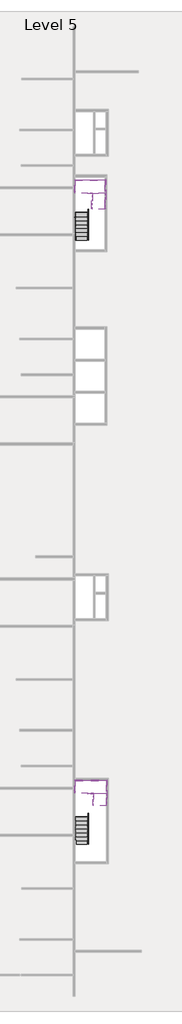
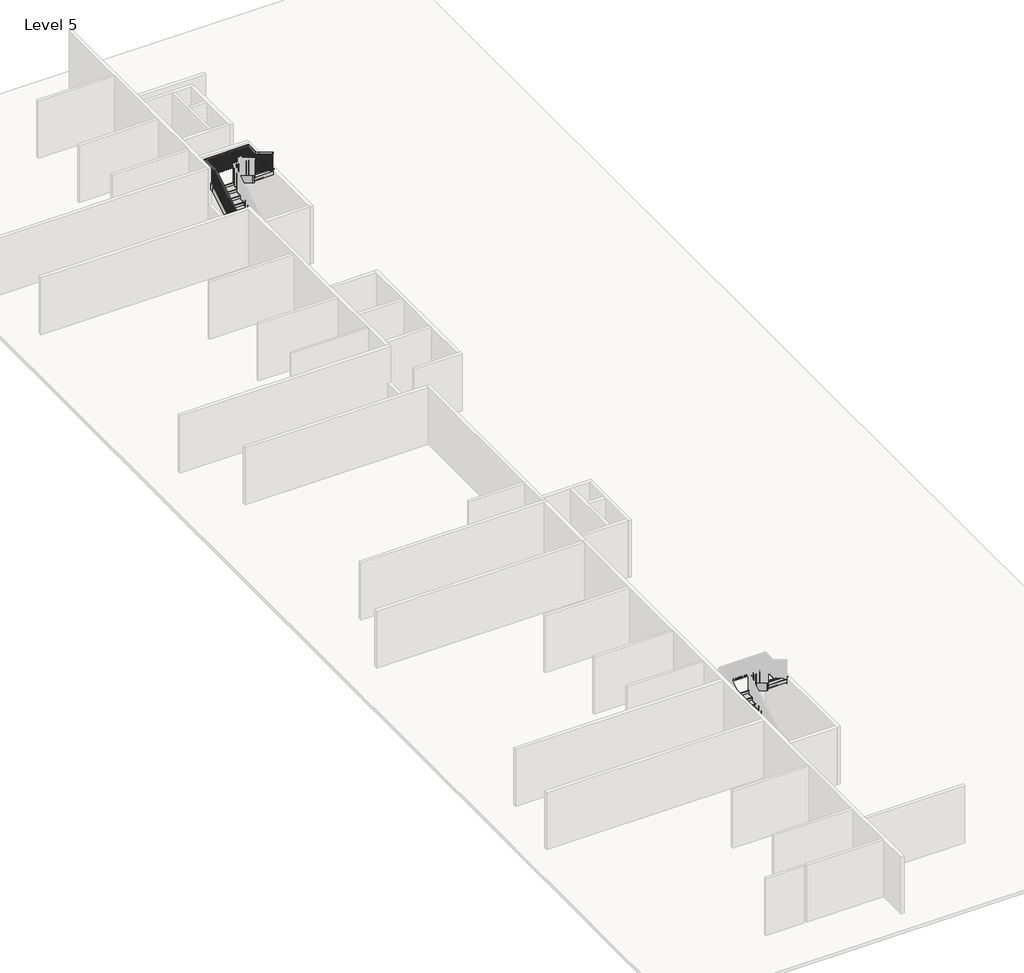
# One storey, part 8 of 8: 16 members, 4 stair flights, 2 slabs, 1 railing.
"""IFC4 building model written with IfcOpenShell, lengths in millimetres."""

from ifc_helpers import new_model, si_unit, frame, origin, place, context, project, spatial, polyline, outline, extrude, faceted_brep, transform, mapped, element, save
from components import non_monolithic_landing_1beb21ea, non_monolithic_landing_abd20321, stair_flight_c80e62dd, stair_flight_f3376f64, stair_flight_9c09f5e7, stair_flight_7705a6e8

model = new_model("IFC4")

# Units and contexts
model_context = context("Model", 3, world=origin())
ifc_project = project(units=[si_unit("LENGTHUNIT", "METRE", prefix="MILLI")], contexts=[model_context])

# Site, building, storey
site = spatial("IfcSite", under=ifc_project)
building = spatial("IfcBuilding", under=site)
storey = spatial("IfcBuildingStorey", under=building, Name="Level 5", Elevation=37426.6172466)

# Members
placement = place(None, origin())
element("IfcMember", 1, ObjectType="Stringer - 2\" Width", at=placement, inside=storey, context=model_context, shape_type="SweptSolid", body=[
    extrude(outline(polyline([(-23154.3851539, 37426.6172466), (-23154.3851539, 37638.7317586), (-19467.0440987, 39873.4839133), (-19381.8896422, 39568.6839133), (-22916.2996422, 37426.6172466), (-23154.3851539, 37426.6172466)])), frame((-3668.2415084, 0.0, 0.0), z_axis=(1.0, 0.0, 0.0), x_axis=(0.0, 1.0, 0.0)), (0.0, 0.0, 1.0), 50.8),
])
element("IfcMember", 2, ObjectType="Stringer - 2\" Width", at=placement, inside=storey, context=model_context, shape_type="SweptSolid", body=[
    extrude(outline(polyline([(-23154.3851539, 37426.6172466), (-23154.3851539, 37638.7317586), (-19572.9851539, 39809.2772131), (-19572.9851539, 39452.8684516), (-22916.2996422, 37426.6172466), (-23154.3851539, 37426.6172466)])), frame((-2703.0415084, 0.0, 0.0), z_axis=(1.0, 0.0, 0.0), x_axis=(0.0, 1.0, 0.0)), (0.0, 0.0, 1.0), 50.8),
])
element("IfcMember", 3, ObjectType="Stringer - 2\" Width", at=placement, inside=storey, context=model_context, shape_type="SweptSolid", body=[
    extrude(outline(polyline([(-19297.9262092, 39873.4839133), (-19383.0806657, 39568.6839133), (-20360.3851539, 40160.9896637), (-20360.3851539, 40517.3984252), (-19297.9262092, 39873.4839133)])), frame((-1382.2415084, 0.0, 0.0), z_axis=(1.0, 0.0, 0.0), x_axis=(0.0, 1.0, 0.0)), (0.0, 0.0, 1.0), 50.8),
])
element("IfcMember", 4, ObjectType="Stringer - 2\" Width", at=placement, inside=storey, context=model_context, shape_type="SweptSolid", body=[
    extrude(outline(polyline([(-19522.1851539, 40009.3984252), (-19522.1851539, 39652.9896637), (-20360.3851539, 40160.9896637), (-20360.3851539, 40517.3984252), (-19522.1851539, 40009.3984252)])), frame((-2347.4415084, 0.0, 0.0), z_axis=(1.0, 0.0, 0.0), x_axis=(0.0, 1.0, 0.0)), (0.0, 0.0, 1.0), 50.8),
])
element("IfcMember", 5, ObjectType="Stringer - 2\" Width", at=placement, inside=storey, context=model_context, shape_type="Brep", body=[
    faceted_brep([(-1382.2415084, -19297.9262092, 39873.4839133), (-1331.4415084, -19297.9262092, 39873.4839133), (-1331.4415084, -18556.9851539, 39873.4839133), (-1382.2415084, -18607.7851539, 39873.4839133), (-1382.2415084, -19383.0806657, 39568.6839133), (-1382.2415084, -18607.7851539, 39568.6839133), (-1331.4415084, -19383.0806657, 39568.6839133), (-1331.4415084, -18556.9851539, 39568.6839133)], [[[0, 1, 2, 3]], [[4, 0, 3, 5]], [[6, 4, 5, 7]], [[1, 6, 7, 2]], [[1, 0, 4, 6]], [[2, 7, 5, 3]]]),
])
element("IfcMember", 6, ObjectType="Stringer - 2\" Width", at=placement, inside=storey, context=model_context, shape_type="SweptSolid", body=[
    extrude(outline(polyline([(-1331.4415084, -18556.9851539), (-1382.2415084, -18607.7851539), (-3617.4415084, -18607.7851539), (-3668.2415084, -18556.9851539), (-1331.4415084, -18556.9851539)])), frame((0.0, 0.0, 39568.6839133), z_axis=(0.0, 0.0, 1.0), x_axis=(1.0, 0.0, 0.0)), (0.0, 0.0, 1.0), 304.8),
])
element("IfcMember", 7, ObjectType="Stringer - 2\" Width", at=placement, inside=storey, context=model_context, shape_type="Brep", body=[
    faceted_brep([(-3617.4415084, -18607.7851539, 39873.4839133), (-3668.2415084, -18556.9851539, 39873.4839133), (-3668.2415084, -19467.0440987, 39873.4839133), (-3617.4415084, -19467.0440987, 39873.4839133), (-3617.4415084, -18607.7851539, 39568.6839133), (-3617.4415084, -19381.8896422, 39568.6839133), (-3668.2415084, -18556.9851539, 39568.6839133), (-3668.2415084, -19381.8896422, 39568.6839133)], [[[0, 1, 2, 3]], [[4, 0, 3, 5]], [[6, 4, 5, 7]], [[1, 6, 7, 2]], [[1, 0, 4, 6]], [[2, 7, 5, 3]]]),
])
element("IfcMember", 8, ObjectType="Stringer - 2\" Width", at=placement, inside=storey, context=model_context, shape_type="SweptSolid", body=[
    extrude(outline(polyline([(-2703.0415084, -19572.9851539), (-2703.0415084, -19522.1851539), (-2347.4415084, -19522.1851539), (-2347.4415084, -19572.9851539), (-2703.0415084, -19572.9851539)])), frame((0.0, 0.0, 39568.6839133), z_axis=(0.0, 0.0, 1.0), x_axis=(1.0, 0.0, 0.0)), (0.0, 0.0, 1.0), 304.8),
])
element("IfcMember", 9, ObjectType="Stringer - 2\" Width", at=placement, inside=storey, context=model_context, shape_type="SweptSolid", body=[
    extrude(outline(polyline([(19841.9216096, 37426.6172466), (19841.9216096, 37638.7317586), (23249.8626649, 39704.1505799), (23335.0171214, 39399.3505799), (20080.0071214, 37426.6172466), (19841.9216096, 37426.6172466)])), frame((-3668.2415084, 0.0, 0.0), z_axis=(1.0, 0.0, 0.0), x_axis=(0.0, 1.0, 0.0)), (0.0, 0.0, 1.0), 50.8),
])
element("IfcMember", 10, ObjectType="Stringer - 2\" Width", at=placement, inside=storey, context=model_context, shape_type="SweptSolid", body=[
    extrude(outline(polyline([(19841.9216096, 37426.6172466), (19841.9216096, 37638.7317586), (23143.9216096, 39639.9438798), (23143.9216096, 39283.5351183), (20080.0071214, 37426.6172466), (19841.9216096, 37426.6172466)])), frame((-2703.0415084, 0.0, 0.0), z_axis=(1.0, 0.0, 0.0), x_axis=(0.0, 1.0, 0.0)), (0.0, 0.0, 1.0), 50.8),
])
element("IfcMember", 11, ObjectType="Stringer - 2\" Width", at=placement, inside=storey, context=model_context, shape_type="SweptSolid", body=[
    extrude(outline(polyline([(23418.9805543, 39704.1505799), (23333.8260978, 39399.3505799), (22077.1216096, 40160.9896637), (22077.1216096, 40517.3984252), (23418.9805543, 39704.1505799)])), frame((-1483.8415084, 0.0, 0.0), z_axis=(1.0, 0.0, 0.0), x_axis=(0.0, 1.0, 0.0)), (0.0, 0.0, 1.0), 50.8),
])
element("IfcMember", 12, ObjectType="Stringer - 2\" Width", at=placement, inside=storey, context=model_context, shape_type="SweptSolid", body=[
    extrude(outline(polyline([(23194.7216096, 39840.0650919), (23194.7216096, 39483.6563304), (22077.1216096, 40160.9896637), (22077.1216096, 40517.3984252), (23194.7216096, 39840.0650919)])), frame((-2449.0415084, 0.0, 0.0), z_axis=(1.0, 0.0, 0.0), x_axis=(0.0, 1.0, 0.0)), (0.0, 0.0, 1.0), 50.8),
])
element("IfcMember", 13, ObjectType="Stringer - 2\" Width", at=placement, inside=storey, context=model_context, shape_type="Brep", body=[
    faceted_brep([(-1483.8415084, 23418.9805543, 39704.1505799), (-1433.0415084, 23418.9805543, 39704.1505799), (-1433.0415084, 24159.9216096, 39704.1505799), (-1483.8415084, 24109.1216096, 39704.1505799), (-1483.8415084, 23333.8260978, 39399.3505799), (-1483.8415084, 24109.1216096, 39399.3505799), (-1433.0415084, 23333.8260978, 39399.3505799), (-1433.0415084, 24159.9216096, 39399.3505799)], [[[0, 1, 2, 3]], [[4, 0, 3, 5]], [[6, 4, 5, 7]], [[1, 6, 7, 2]], [[1, 0, 4, 6]], [[2, 7, 5, 3]]]),
])
element("IfcMember", 14, ObjectType="Stringer - 2\" Width", at=placement, inside=storey, context=model_context, shape_type="SweptSolid", body=[
    extrude(outline(polyline([(-1433.0415084, 24159.9216096), (-1483.8415084, 24109.1216096), (-3617.4415084, 24109.1216096), (-3668.2415084, 24159.9216096), (-1433.0415084, 24159.9216096)])), frame((0.0, 0.0, 39399.3505799), z_axis=(0.0, 0.0, 1.0), x_axis=(1.0, 0.0, 0.0)), (0.0, 0.0, 1.0), 304.8),
])
element("IfcMember", 15, ObjectType="Stringer - 2\" Width", at=placement, inside=storey, context=model_context, shape_type="Brep", body=[
    faceted_brep([(-3617.4415084, 24109.1216096, 39704.1505799), (-3668.2415084, 24159.9216096, 39704.1505799), (-3668.2415084, 23249.8626649, 39704.1505799), (-3617.4415084, 23249.8626649, 39704.1505799), (-3617.4415084, 24109.1216096, 39399.3505799), (-3617.4415084, 23335.0171214, 39399.3505799), (-3668.2415084, 24159.9216096, 39399.3505799), (-3668.2415084, 23335.0171214, 39399.3505799)], [[[0, 1, 2, 3]], [[4, 0, 3, 5]], [[6, 4, 5, 7]], [[1, 6, 7, 2]], [[1, 0, 4, 6]], [[2, 7, 5, 3]]]),
])
element("IfcMember", 16, ObjectType="Stringer - 2\" Width", at=placement, inside=storey, context=model_context, shape_type="SweptSolid", body=[
    extrude(outline(polyline([(-2703.0415084, 23143.9216096), (-2703.0415084, 23194.7216096), (-2449.0415084, 23194.7216096), (-2449.0415084, 23143.9216096), (-2703.0415084, 23143.9216096)])), frame((0.0, 0.0, 39399.3505799), z_axis=(0.0, 0.0, 1.0), x_axis=(1.0, 0.0, 0.0)), (0.0, 0.0, 1.0), 304.8),
])

# Railing
element("IfcRailing", 17, ObjectType="Handrail - Rectangular", at=placement, inside=storey, context=model_context, shape_type="SolidModel", body=[
    faceted_brep([(-3617.4415084, 19841.9216096, 38510.3505799), (-3617.4415084, 19841.9216096, 38450.9491197), (-3566.6415084, 19841.9216096, 38450.9491197), (-3566.6415084, 19841.9216096, 38510.3505799), (-3617.4415084, 23194.7216096, 40542.3505799), (-3617.4415084, 23208.914019, 40491.5505799), (-3566.6415084, 23208.914019, 40491.5505799), (-3566.6415084, 23194.7216096, 40542.3505799), (-3617.4415084, 24109.1216096, 40542.3505799), (-3617.4415084, 24109.1216096, 40491.5505799), (-3566.6415084, 24058.3216096, 40491.5505799), (-3566.6415084, 24058.3216096, 40542.3505799), (-1483.8415084, 24109.1216096, 40542.3505799), (-1483.8415084, 24109.1216096, 40491.5505799), (-1534.6415084, 24058.3216096, 40491.5505799), (-1534.6415084, 24058.3216096, 40542.3505799), (-1483.8415084, 23474.1216096, 40542.3505799), (-1483.8415084, 23459.9292002, 40491.5505799), (-1534.6415084, 23459.9292002, 40491.5505799), (-1534.6415084, 23474.1216096, 40542.3505799), (-1483.8415084, 23194.7216096, 40711.6839133), (-1483.8415084, 23168.3918824, 40668.2398634), (-1534.6415084, 23168.3918824, 40668.2398634), (-1534.6415084, 23194.7216096, 40711.6839133), (-1483.8415084, 22077.1216096, 41389.0172466), (-1534.6415084, 22077.1216096, 41389.0172466), (-1534.6415084, 22077.1216096, 41329.6157863), (-1483.8415084, 22077.1216096, 41329.6157863)], [[[0, 1, 2, 3]], [[1, 0, 4, 5]], [[2, 1, 5, 6]], [[3, 2, 6, 7]], [[0, 3, 7, 4]], [[5, 4, 8, 9]], [[6, 5, 9, 10]], [[7, 6, 10, 11]], [[4, 7, 11, 8]], [[9, 8, 12, 13]], [[10, 9, 13, 14]], [[11, 10, 14, 15]], [[8, 11, 15, 12]], [[13, 12, 16, 17]], [[14, 13, 17, 18]], [[15, 14, 18, 19]], [[12, 15, 19, 16]], [[17, 16, 20, 21]], [[18, 17, 21, 22]], [[19, 18, 22, 23]], [[16, 19, 23, 20]], [[24, 25, 26, 27]], [[21, 20, 24, 27]], [[22, 21, 27, 26]], [[23, 22, 26, 25]], [[20, 23, 25, 24]]]),
    extrude(outline(polyline([(22188.2466096, 41262.2673015), (22188.2466096, 40305.2839133), (22169.1966096, 40305.2839133), (22169.1966096, 41273.812756), (22188.2466096, 41262.2673015)])), frame((-1518.7665084, 0.0, 0.0), z_axis=(1.0, 0.0, 0.0), x_axis=(0.0, 1.0, 0.0)), (0.0, 0.0, 1.0), 19.05),
    extrude(outline(polyline([(22289.8466096, 41200.6915439), (22289.8466096, 40305.2839133), (22270.7966096, 40305.2839133), (22270.7966096, 41212.2369985), (22289.8466096, 41200.6915439)])), frame((-1518.7665084, 0.0, 0.0), z_axis=(1.0, 0.0, 0.0), x_axis=(0.0, 1.0, 0.0)), (0.0, 0.0, 1.0), 19.05),
    extrude(outline(polyline([(22391.4466096, 41139.1157863), (22391.4466096, 40135.9505799), (22372.3966096, 40135.9505799), (22372.3966096, 41150.6612409), (22391.4466096, 41139.1157863)])), frame((-1518.7665084, 0.0, 0.0), z_axis=(1.0, 0.0, 0.0), x_axis=(0.0, 1.0, 0.0)), (0.0, 0.0, 1.0), 19.05),
    extrude(outline(polyline([(22493.0466096, 41077.5400288), (22493.0466096, 40135.9505799), (22473.9966096, 40135.9505799), (22473.9966096, 41089.0854833), (22493.0466096, 41077.5400288)])), frame((-1518.7665084, 0.0, 0.0), z_axis=(1.0, 0.0, 0.0), x_axis=(0.0, 1.0, 0.0)), (0.0, 0.0, 1.0), 19.05),
    extrude(outline(polyline([(22594.6466096, 41015.9642712), (22594.6466096, 40135.9505799), (22575.5966096, 40135.9505799), (22575.5966096, 41027.5097257), (22594.6466096, 41015.9642712)])), frame((-1518.7665084, 0.0, 0.0), z_axis=(1.0, 0.0, 0.0), x_axis=(0.0, 1.0, 0.0)), (0.0, 0.0, 1.0), 19.05),
    extrude(outline(polyline([(22696.2466096, 40954.3885136), (22696.2466096, 39966.6172466), (22677.1966096, 39966.6172466), (22677.1966096, 40965.9339682), (22696.2466096, 40954.3885136)])), frame((-1518.7665084, 0.0, 0.0), z_axis=(1.0, 0.0, 0.0), x_axis=(0.0, 1.0, 0.0)), (0.0, 0.0, 1.0), 19.05),
    extrude(outline(polyline([(22797.8466096, 40892.812756), (22797.8466096, 39966.6172466), (22778.7966096, 39966.6172466), (22778.7966096, 40904.3582106), (22797.8466096, 40892.812756)])), frame((-1518.7665084, 0.0, 0.0), z_axis=(1.0, 0.0, 0.0), x_axis=(0.0, 1.0, 0.0)), (0.0, 0.0, 1.0), 19.05),
    extrude(outline(polyline([(22899.4466096, 40831.2369985), (22899.4466096, 39966.6172466), (22880.3966096, 39966.6172466), (22880.3966096, 40842.782453), (22899.4466096, 40831.2369985)])), frame((-1518.7665084, 0.0, 0.0), z_axis=(1.0, 0.0, 0.0), x_axis=(0.0, 1.0, 0.0)), (0.0, 0.0, 1.0), 19.05),
    extrude(outline(polyline([(23001.0466096, 40769.6612409), (23001.0466096, 39797.2839133), (22981.9966096, 39797.2839133), (22981.9966096, 40781.2066954), (23001.0466096, 40769.6612409)])), frame((-1518.7665084, 0.0, 0.0), z_axis=(1.0, 0.0, 0.0), x_axis=(0.0, 1.0, 0.0)), (0.0, 0.0, 1.0), 19.05),
    extrude(outline(polyline([(23102.6466096, 40708.0854833), (23102.6466096, 39797.2839133), (23083.5966096, 39797.2839133), (23083.5966096, 40719.6309379), (23102.6466096, 40708.0854833)])), frame((-1518.7665084, 0.0, 0.0), z_axis=(1.0, 0.0, 0.0), x_axis=(0.0, 1.0, 0.0)), (0.0, 0.0, 1.0), 19.05),
    extrude(outline(polyline([(23280.4466096, 40600.3279076), (23280.4466096, 39627.9505799), (23261.3966096, 39627.9505799), (23261.3966096, 40611.8733621), (23280.4466096, 40600.3279076)])), frame((-1518.7665084, 0.0, 0.0), z_axis=(1.0, 0.0, 0.0), x_axis=(0.0, 1.0, 0.0)), (0.0, 0.0, 1.0), 19.05),
    extrude(outline(polyline([(23382.0466096, 40538.75215), (23382.0466096, 39627.9505799), (23362.9966096, 39627.9505799), (23362.9966096, 40550.2976045), (23382.0466096, 40538.75215)])), frame((-1518.7665084, 0.0, 0.0), z_axis=(1.0, 0.0, 0.0), x_axis=(0.0, 1.0, 0.0)), (0.0, 0.0, 1.0), 19.05),
    extrude(outline(polyline([(-1499.7165084, 23483.6466096), (-1499.7165084, 23464.5966096), (-1518.7665084, 23464.5966096), (-1518.7665084, 23483.6466096), (-1499.7165084, 23483.6466096)])), frame((0.0, 0.0, 39627.9505799), z_axis=(0.0, 0.0, 1.0), x_axis=(1.0, 0.0, 0.0)), (0.0, 0.0, 1.0), 863.6),
    extrude(outline(polyline([(-1499.7165084, 23585.2466096), (-1499.7165084, 23566.1966096), (-1518.7665084, 23566.1966096), (-1518.7665084, 23585.2466096), (-1499.7165084, 23585.2466096)])), frame((0.0, 0.0, 39627.9505799), z_axis=(0.0, 0.0, 1.0), x_axis=(1.0, 0.0, 0.0)), (0.0, 0.0, 1.0), 863.6),
    extrude(outline(polyline([(-1499.7165084, 23686.8466096), (-1499.7165084, 23667.7966096), (-1518.7665084, 23667.7966096), (-1518.7665084, 23686.8466096), (-1499.7165084, 23686.8466096)])), frame((0.0, 0.0, 39627.9505799), z_axis=(0.0, 0.0, 1.0), x_axis=(1.0, 0.0, 0.0)), (0.0, 0.0, 1.0), 863.6),
    extrude(outline(polyline([(-1499.7165084, 23788.4466096), (-1499.7165084, 23769.3966096), (-1518.7665084, 23769.3966096), (-1518.7665084, 23788.4466096), (-1499.7165084, 23788.4466096)])), frame((0.0, 0.0, 39627.9505799), z_axis=(0.0, 0.0, 1.0), x_axis=(1.0, 0.0, 0.0)), (0.0, 0.0, 1.0), 863.6),
    extrude(outline(polyline([(-1499.7165084, 23890.0466096), (-1499.7165084, 23870.9966096), (-1518.7665084, 23870.9966096), (-1518.7665084, 23890.0466096), (-1499.7165084, 23890.0466096)])), frame((0.0, 0.0, 39627.9505799), z_axis=(0.0, 0.0, 1.0), x_axis=(1.0, 0.0, 0.0)), (0.0, 0.0, 1.0), 863.6),
    extrude(outline(polyline([(-1499.7165084, 23991.6466096), (-1499.7165084, 23972.5966096), (-1518.7665084, 23972.5966096), (-1518.7665084, 23991.6466096), (-1499.7165084, 23991.6466096)])), frame((0.0, 0.0, 39627.9505799), z_axis=(0.0, 0.0, 1.0), x_axis=(1.0, 0.0, 0.0)), (0.0, 0.0, 1.0), 863.6),
    extrude(outline(polyline([(-1569.5665084, 24093.2466096), (-1550.5165084, 24093.2466096), (-1550.5165084, 24074.1966096), (-1569.5665084, 24074.1966096), (-1569.5665084, 24093.2466096)])), frame((0.0, 0.0, 39627.9505799), z_axis=(0.0, 0.0, 1.0), x_axis=(1.0, 0.0, 0.0)), (0.0, 0.0, 1.0), 863.6),
    extrude(outline(polyline([(-1671.1665084, 24093.2466096), (-1652.1165084, 24093.2466096), (-1652.1165084, 24074.1966096), (-1671.1665084, 24074.1966096), (-1671.1665084, 24093.2466096)])), frame((0.0, 0.0, 39627.9505799), z_axis=(0.0, 0.0, 1.0), x_axis=(1.0, 0.0, 0.0)), (0.0, 0.0, 1.0), 863.6),
    extrude(outline(polyline([(-1772.7665084, 24093.2466096), (-1753.7165084, 24093.2466096), (-1753.7165084, 24074.1966096), (-1772.7665084, 24074.1966096), (-1772.7665084, 24093.2466096)])), frame((0.0, 0.0, 39627.9505799), z_axis=(0.0, 0.0, 1.0), x_axis=(1.0, 0.0, 0.0)), (0.0, 0.0, 1.0), 863.6),
    extrude(outline(polyline([(-1874.3665084, 24093.2466096), (-1855.3165084, 24093.2466096), (-1855.3165084, 24074.1966096), (-1874.3665084, 24074.1966096), (-1874.3665084, 24093.2466096)])), frame((0.0, 0.0, 39627.9505799), z_axis=(0.0, 0.0, 1.0), x_axis=(1.0, 0.0, 0.0)), (0.0, 0.0, 1.0), 863.6),
    extrude(outline(polyline([(-1975.9665084, 24093.2466096), (-1956.9165084, 24093.2466096), (-1956.9165084, 24074.1966096), (-1975.9665084, 24074.1966096), (-1975.9665084, 24093.2466096)])), frame((0.0, 0.0, 39627.9505799), z_axis=(0.0, 0.0, 1.0), x_axis=(1.0, 0.0, 0.0)), (0.0, 0.0, 1.0), 863.6),
    extrude(outline(polyline([(-2077.5665084, 24093.2466096), (-2058.5165084, 24093.2466096), (-2058.5165084, 24074.1966096), (-2077.5665084, 24074.1966096), (-2077.5665084, 24093.2466096)])), frame((0.0, 0.0, 39627.9505799), z_axis=(0.0, 0.0, 1.0), x_axis=(1.0, 0.0, 0.0)), (0.0, 0.0, 1.0), 863.6),
    extrude(outline(polyline([(-2179.1665084, 24093.2466096), (-2160.1165084, 24093.2466096), (-2160.1165084, 24074.1966096), (-2179.1665084, 24074.1966096), (-2179.1665084, 24093.2466096)])), frame((0.0, 0.0, 39627.9505799), z_axis=(0.0, 0.0, 1.0), x_axis=(1.0, 0.0, 0.0)), (0.0, 0.0, 1.0), 863.6),
    extrude(outline(polyline([(-2280.7665084, 24093.2466096), (-2261.7165084, 24093.2466096), (-2261.7165084, 24074.1966096), (-2280.7665084, 24074.1966096), (-2280.7665084, 24093.2466096)])), frame((0.0, 0.0, 39627.9505799), z_axis=(0.0, 0.0, 1.0), x_axis=(1.0, 0.0, 0.0)), (0.0, 0.0, 1.0), 863.6),
    extrude(outline(polyline([(-2382.3665084, 24093.2466096), (-2363.3165084, 24093.2466096), (-2363.3165084, 24074.1966096), (-2382.3665084, 24074.1966096), (-2382.3665084, 24093.2466096)])), frame((0.0, 0.0, 39627.9505799), z_axis=(0.0, 0.0, 1.0), x_axis=(1.0, 0.0, 0.0)), (0.0, 0.0, 1.0), 863.6),
    extrude(outline(polyline([(-2483.9665084, 24093.2466096), (-2464.9165084, 24093.2466096), (-2464.9165084, 24074.1966096), (-2483.9665084, 24074.1966096), (-2483.9665084, 24093.2466096)])), frame((0.0, 0.0, 39627.9505799), z_axis=(0.0, 0.0, 1.0), x_axis=(1.0, 0.0, 0.0)), (0.0, 0.0, 1.0), 863.6),
    extrude(outline(polyline([(-2585.5665084, 24093.2466096), (-2566.5165084, 24093.2466096), (-2566.5165084, 24074.1966096), (-2585.5665084, 24074.1966096), (-2585.5665084, 24093.2466096)])), frame((0.0, 0.0, 39627.9505799), z_axis=(0.0, 0.0, 1.0), x_axis=(1.0, 0.0, 0.0)), (0.0, 0.0, 1.0), 863.6),
    extrude(outline(polyline([(-2687.1665084, 24093.2466096), (-2668.1165084, 24093.2466096), (-2668.1165084, 24074.1966096), (-2687.1665084, 24074.1966096), (-2687.1665084, 24093.2466096)])), frame((0.0, 0.0, 39627.9505799), z_axis=(0.0, 0.0, 1.0), x_axis=(1.0, 0.0, 0.0)), (0.0, 0.0, 1.0), 863.6),
    extrude(outline(polyline([(-2788.7665084, 24093.2466096), (-2769.7165084, 24093.2466096), (-2769.7165084, 24074.1966096), (-2788.7665084, 24074.1966096), (-2788.7665084, 24093.2466096)])), frame((0.0, 0.0, 39627.9505799), z_axis=(0.0, 0.0, 1.0), x_axis=(1.0, 0.0, 0.0)), (0.0, 0.0, 1.0), 863.6),
    extrude(outline(polyline([(-2890.3665084, 24093.2466096), (-2871.3165084, 24093.2466096), (-2871.3165084, 24074.1966096), (-2890.3665084, 24074.1966096), (-2890.3665084, 24093.2466096)])), frame((0.0, 0.0, 39627.9505799), z_axis=(0.0, 0.0, 1.0), x_axis=(1.0, 0.0, 0.0)), (0.0, 0.0, 1.0), 863.6),
    extrude(outline(polyline([(-2991.9665084, 24093.2466096), (-2972.9165084, 24093.2466096), (-2972.9165084, 24074.1966096), (-2991.9665084, 24074.1966096), (-2991.9665084, 24093.2466096)])), frame((0.0, 0.0, 39627.9505799), z_axis=(0.0, 0.0, 1.0), x_axis=(1.0, 0.0, 0.0)), (0.0, 0.0, 1.0), 863.6),
    extrude(outline(polyline([(-3093.5665084, 24093.2466096), (-3074.5165084, 24093.2466096), (-3074.5165084, 24074.1966096), (-3093.5665084, 24074.1966096), (-3093.5665084, 24093.2466096)])), frame((0.0, 0.0, 39627.9505799), z_axis=(0.0, 0.0, 1.0), x_axis=(1.0, 0.0, 0.0)), (0.0, 0.0, 1.0), 863.6),
    extrude(outline(polyline([(-3195.1665084, 24093.2466096), (-3176.1165084, 24093.2466096), (-3176.1165084, 24074.1966096), (-3195.1665084, 24074.1966096), (-3195.1665084, 24093.2466096)])), frame((0.0, 0.0, 39627.9505799), z_axis=(0.0, 0.0, 1.0), x_axis=(1.0, 0.0, 0.0)), (0.0, 0.0, 1.0), 863.6),
    extrude(outline(polyline([(-3296.7665084, 24093.2466096), (-3277.7165084, 24093.2466096), (-3277.7165084, 24074.1966096), (-3296.7665084, 24074.1966096), (-3296.7665084, 24093.2466096)])), frame((0.0, 0.0, 39627.9505799), z_axis=(0.0, 0.0, 1.0), x_axis=(1.0, 0.0, 0.0)), (0.0, 0.0, 1.0), 863.6),
    extrude(outline(polyline([(-3398.3665084, 24093.2466096), (-3379.3165084, 24093.2466096), (-3379.3165084, 24074.1966096), (-3398.3665084, 24074.1966096), (-3398.3665084, 24093.2466096)])), frame((0.0, 0.0, 39627.9505799), z_axis=(0.0, 0.0, 1.0), x_axis=(1.0, 0.0, 0.0)), (0.0, 0.0, 1.0), 863.6),
    extrude(outline(polyline([(-3499.9665084, 24093.2466096), (-3480.9165084, 24093.2466096), (-3480.9165084, 24074.1966096), (-3499.9665084, 24074.1966096), (-3499.9665084, 24093.2466096)])), frame((0.0, 0.0, 39627.9505799), z_axis=(0.0, 0.0, 1.0), x_axis=(1.0, 0.0, 0.0)), (0.0, 0.0, 1.0), 863.6),
    extrude(outline(polyline([(-3601.5665084, 23997.9966096), (-3601.5665084, 24017.0466096), (-3582.5165084, 24017.0466096), (-3582.5165084, 23997.9966096), (-3601.5665084, 23997.9966096)])), frame((0.0, 0.0, 39627.9505799), z_axis=(0.0, 0.0, 1.0), x_axis=(1.0, 0.0, 0.0)), (0.0, 0.0, 1.0), 863.6),
    extrude(outline(polyline([(-3601.5665084, 23896.3966096), (-3601.5665084, 23915.4466096), (-3582.5165084, 23915.4466096), (-3582.5165084, 23896.3966096), (-3601.5665084, 23896.3966096)])), frame((0.0, 0.0, 39627.9505799), z_axis=(0.0, 0.0, 1.0), x_axis=(1.0, 0.0, 0.0)), (0.0, 0.0, 1.0), 863.6),
    extrude(outline(polyline([(-3601.5665084, 23794.7966096), (-3601.5665084, 23813.8466096), (-3582.5165084, 23813.8466096), (-3582.5165084, 23794.7966096), (-3601.5665084, 23794.7966096)])), frame((0.0, 0.0, 39627.9505799), z_axis=(0.0, 0.0, 1.0), x_axis=(1.0, 0.0, 0.0)), (0.0, 0.0, 1.0), 863.6),
    extrude(outline(polyline([(-3601.5665084, 23693.1966096), (-3601.5665084, 23712.2466096), (-3582.5165084, 23712.2466096), (-3582.5165084, 23693.1966096), (-3601.5665084, 23693.1966096)])), frame((0.0, 0.0, 39627.9505799), z_axis=(0.0, 0.0, 1.0), x_axis=(1.0, 0.0, 0.0)), (0.0, 0.0, 1.0), 863.6),
    extrude(outline(polyline([(-3601.5665084, 23591.5966096), (-3601.5665084, 23610.6466096), (-3582.5165084, 23610.6466096), (-3582.5165084, 23591.5966096), (-3601.5665084, 23591.5966096)])), frame((0.0, 0.0, 39627.9505799), z_axis=(0.0, 0.0, 1.0), x_axis=(1.0, 0.0, 0.0)), (0.0, 0.0, 1.0), 863.6),
    extrude(outline(polyline([(-3601.5665084, 23489.9966096), (-3601.5665084, 23509.0466096), (-3582.5165084, 23509.0466096), (-3582.5165084, 23489.9966096), (-3601.5665084, 23489.9966096)])), frame((0.0, 0.0, 39627.9505799), z_axis=(0.0, 0.0, 1.0), x_axis=(1.0, 0.0, 0.0)), (0.0, 0.0, 1.0), 863.6),
    extrude(outline(polyline([(-3601.5665084, 23388.3966096), (-3601.5665084, 23407.4466096), (-3582.5165084, 23407.4466096), (-3582.5165084, 23388.3966096), (-3601.5665084, 23388.3966096)])), frame((0.0, 0.0, 39627.9505799), z_axis=(0.0, 0.0, 1.0), x_axis=(1.0, 0.0, 0.0)), (0.0, 0.0, 1.0), 863.6),
    extrude(outline(polyline([(-3601.5665084, 23286.7966096), (-3601.5665084, 23305.8466096), (-3582.5165084, 23305.8466096), (-3582.5165084, 23286.7966096), (-3601.5665084, 23286.7966096)])), frame((0.0, 0.0, 39627.9505799), z_axis=(0.0, 0.0, 1.0), x_axis=(1.0, 0.0, 0.0)), (0.0, 0.0, 1.0), 863.6),
    extrude(outline(polyline([(23102.6466096, 40427.1460894), (23102.6466096, 39458.6172466), (23083.5966096, 39458.6172466), (23083.5966096, 40415.6006348), (23102.6466096, 40427.1460894)])), frame((-3601.5665084, 0.0, 0.0), z_axis=(1.0, 0.0, 0.0), x_axis=(0.0, 1.0, 0.0)), (0.0, 0.0, 1.0), 19.05),
    extrude(outline(polyline([(23001.0466096, 40365.5703318), (23001.0466096, 39458.6172466), (22981.9966096, 39458.6172466), (22981.9966096, 40354.0248773), (23001.0466096, 40365.5703318)])), frame((-3601.5665084, 0.0, 0.0), z_axis=(1.0, 0.0, 0.0), x_axis=(0.0, 1.0, 0.0)), (0.0, 0.0, 1.0), 19.05),
    extrude(outline(polyline([(22899.4466096, 40303.9945742), (22899.4466096, 39289.2839133), (22880.3966096, 39289.2839133), (22880.3966096, 40292.4491197), (22899.4466096, 40303.9945742)])), frame((-3601.5665084, 0.0, 0.0), z_axis=(1.0, 0.0, 0.0), x_axis=(0.0, 1.0, 0.0)), (0.0, 0.0, 1.0), 19.05),
    extrude(outline(polyline([(22797.8466096, 40242.4188166), (22797.8466096, 39289.2839133), (22778.7966096, 39289.2839133), (22778.7966096, 40230.8733621), (22797.8466096, 40242.4188166)])), frame((-3601.5665084, 0.0, 0.0), z_axis=(1.0, 0.0, 0.0), x_axis=(0.0, 1.0, 0.0)), (0.0, 0.0, 1.0), 19.05),
    extrude(outline(polyline([(22696.2466096, 40180.8430591), (22696.2466096, 39289.2839133), (22677.1966096, 39289.2839133), (22677.1966096, 40169.2976045), (22696.2466096, 40180.8430591)])), frame((-3601.5665084, 0.0, 0.0), z_axis=(1.0, 0.0, 0.0), x_axis=(0.0, 1.0, 0.0)), (0.0, 0.0, 1.0), 19.05),
    extrude(outline(polyline([(22594.6466096, 40119.2673015), (22594.6466096, 39119.9505799), (22575.5966096, 39119.9505799), (22575.5966096, 40107.721847), (22594.6466096, 40119.2673015)])), frame((-3601.5665084, 0.0, 0.0), z_axis=(1.0, 0.0, 0.0), x_axis=(0.0, 1.0, 0.0)), (0.0, 0.0, 1.0), 19.05),
    extrude(outline(polyline([(22493.0466096, 40057.6915439), (22493.0466096, 39119.9505799), (22473.9966096, 39119.9505799), (22473.9966096, 40046.1460894), (22493.0466096, 40057.6915439)])), frame((-3601.5665084, 0.0, 0.0), z_axis=(1.0, 0.0, 0.0), x_axis=(0.0, 1.0, 0.0)), (0.0, 0.0, 1.0), 19.05),
    extrude(outline(polyline([(22391.4466096, 39996.1157863), (22391.4466096, 39119.9505799), (22372.3966096, 39119.9505799), (22372.3966096, 39984.5703318), (22391.4466096, 39996.1157863)])), frame((-3601.5665084, 0.0, 0.0), z_axis=(1.0, 0.0, 0.0), x_axis=(0.0, 1.0, 0.0)), (0.0, 0.0, 1.0), 19.05),
    extrude(outline(polyline([(22289.8466096, 39934.5400288), (22289.8466096, 38950.6172466), (22270.7966096, 38950.6172466), (22270.7966096, 39922.9945742), (22289.8466096, 39934.5400288)])), frame((-3601.5665084, 0.0, 0.0), z_axis=(1.0, 0.0, 0.0), x_axis=(0.0, 1.0, 0.0)), (0.0, 0.0, 1.0), 19.05),
    extrude(outline(polyline([(22188.2466096, 39872.9642712), (22188.2466096, 38950.6172466), (22169.1966096, 38950.6172466), (22169.1966096, 39861.4188166), (22188.2466096, 39872.9642712)])), frame((-3601.5665084, 0.0, 0.0), z_axis=(1.0, 0.0, 0.0), x_axis=(0.0, 1.0, 0.0)), (0.0, 0.0, 1.0), 19.05),
    extrude(outline(polyline([(22086.6466096, 39811.3885136), (22086.6466096, 38950.6172466), (22067.5966096, 38950.6172466), (22067.5966096, 39799.8430591), (22086.6466096, 39811.3885136)])), frame((-3601.5665084, 0.0, 0.0), z_axis=(1.0, 0.0, 0.0), x_axis=(0.0, 1.0, 0.0)), (0.0, 0.0, 1.0), 19.05),
    extrude(outline(polyline([(21985.0466096, 39749.812756), (21985.0466096, 38781.2839133), (21965.9966096, 38781.2839133), (21965.9966096, 39738.2673015), (21985.0466096, 39749.812756)])), frame((-3601.5665084, 0.0, 0.0), z_axis=(1.0, 0.0, 0.0), x_axis=(0.0, 1.0, 0.0)), (0.0, 0.0, 1.0), 19.05),
    extrude(outline(polyline([(21883.4466096, 39688.2369985), (21883.4466096, 38781.2839133), (21864.3966096, 38781.2839133), (21864.3966096, 39676.6915439), (21883.4466096, 39688.2369985)])), frame((-3601.5665084, 0.0, 0.0), z_axis=(1.0, 0.0, 0.0), x_axis=(0.0, 1.0, 0.0)), (0.0, 0.0, 1.0), 19.05),
    extrude(outline(polyline([(21781.8466096, 39626.6612409), (21781.8466096, 38611.9505799), (21762.7966096, 38611.9505799), (21762.7966096, 39615.1157863), (21781.8466096, 39626.6612409)])), frame((-3601.5665084, 0.0, 0.0), z_axis=(1.0, 0.0, 0.0), x_axis=(0.0, 1.0, 0.0)), (0.0, 0.0, 1.0), 19.05),
    extrude(outline(polyline([(21680.2466096, 39565.0854833), (21680.2466096, 38611.9505799), (21661.1966096, 38611.9505799), (21661.1966096, 39553.5400288), (21680.2466096, 39565.0854833)])), frame((-3601.5665084, 0.0, 0.0), z_axis=(1.0, 0.0, 0.0), x_axis=(0.0, 1.0, 0.0)), (0.0, 0.0, 1.0), 19.05),
    extrude(outline(polyline([(21578.6466096, 39503.5097257), (21578.6466096, 38611.9505799), (21559.5966096, 38611.9505799), (21559.5966096, 39491.9642712), (21578.6466096, 39503.5097257)])), frame((-3601.5665084, 0.0, 0.0), z_axis=(1.0, 0.0, 0.0), x_axis=(0.0, 1.0, 0.0)), (0.0, 0.0, 1.0), 19.05),
    extrude(outline(polyline([(21477.0466096, 39441.9339682), (21477.0466096, 38442.6172466), (21457.9966096, 38442.6172466), (21457.9966096, 39430.3885136), (21477.0466096, 39441.9339682)])), frame((-3601.5665084, 0.0, 0.0), z_axis=(1.0, 0.0, 0.0), x_axis=(0.0, 1.0, 0.0)), (0.0, 0.0, 1.0), 19.05),
    extrude(outline(polyline([(21375.4466096, 39380.3582106), (21375.4466096, 38442.6172466), (21356.3966096, 38442.6172466), (21356.3966096, 39368.812756), (21375.4466096, 39380.3582106)])), frame((-3601.5665084, 0.0, 0.0), z_axis=(1.0, 0.0, 0.0), x_axis=(0.0, 1.0, 0.0)), (0.0, 0.0, 1.0), 19.05),
    extrude(outline(polyline([(21273.8466096, 39318.782453), (21273.8466096, 38442.6172466), (21254.7966096, 38442.6172466), (21254.7966096, 39307.2369985), (21273.8466096, 39318.782453)])), frame((-3601.5665084, 0.0, 0.0), z_axis=(1.0, 0.0, 0.0), x_axis=(0.0, 1.0, 0.0)), (0.0, 0.0, 1.0), 19.05),
    extrude(outline(polyline([(21172.2466096, 39257.2066954), (21172.2466096, 38273.2839133), (21153.1966096, 38273.2839133), (21153.1966096, 39245.6612409), (21172.2466096, 39257.2066954)])), frame((-3601.5665084, 0.0, 0.0), z_axis=(1.0, 0.0, 0.0), x_axis=(0.0, 1.0, 0.0)), (0.0, 0.0, 1.0), 19.05),
    extrude(outline(polyline([(21070.6466096, 39195.6309379), (21070.6466096, 38273.2839133), (21051.5966096, 38273.2839133), (21051.5966096, 39184.0854833), (21070.6466096, 39195.6309379)])), frame((-3601.5665084, 0.0, 0.0), z_axis=(1.0, 0.0, 0.0), x_axis=(0.0, 1.0, 0.0)), (0.0, 0.0, 1.0), 19.05),
    extrude(outline(polyline([(20969.0466096, 39134.0551803), (20969.0466096, 38273.2839133), (20949.9966096, 38273.2839133), (20949.9966096, 39122.5097257), (20969.0466096, 39134.0551803)])), frame((-3601.5665084, 0.0, 0.0), z_axis=(1.0, 0.0, 0.0), x_axis=(0.0, 1.0, 0.0)), (0.0, 0.0, 1.0), 19.05),
    extrude(outline(polyline([(20867.4466096, 39072.4794227), (20867.4466096, 38103.9505799), (20848.3966096, 38103.9505799), (20848.3966096, 39060.9339682), (20867.4466096, 39072.4794227)])), frame((-3601.5665084, 0.0, 0.0), z_axis=(1.0, 0.0, 0.0), x_axis=(0.0, 1.0, 0.0)), (0.0, 0.0, 1.0), 19.05),
    extrude(outline(polyline([(20765.8466096, 39010.9036651), (20765.8466096, 38103.9505799), (20746.7966096, 38103.9505799), (20746.7966096, 38999.3582106), (20765.8466096, 39010.9036651)])), frame((-3601.5665084, 0.0, 0.0), z_axis=(1.0, 0.0, 0.0), x_axis=(0.0, 1.0, 0.0)), (0.0, 0.0, 1.0), 19.05),
    extrude(outline(polyline([(20664.2466096, 38949.3279076), (20664.2466096, 37934.6172466), (20645.1966096, 37934.6172466), (20645.1966096, 38937.782453), (20664.2466096, 38949.3279076)])), frame((-3601.5665084, 0.0, 0.0), z_axis=(1.0, 0.0, 0.0), x_axis=(0.0, 1.0, 0.0)), (0.0, 0.0, 1.0), 19.05),
    extrude(outline(polyline([(20562.6466096, 38887.75215), (20562.6466096, 37934.6172466), (20543.5966096, 37934.6172466), (20543.5966096, 38876.2066954), (20562.6466096, 38887.75215)])), frame((-3601.5665084, 0.0, 0.0), z_axis=(1.0, 0.0, 0.0), x_axis=(0.0, 1.0, 0.0)), (0.0, 0.0, 1.0), 19.05),
    extrude(outline(polyline([(20461.0466096, 38826.1763924), (20461.0466096, 37934.6172466), (20441.9966096, 37934.6172466), (20441.9966096, 38814.6309379), (20461.0466096, 38826.1763924)])), frame((-3601.5665084, 0.0, 0.0), z_axis=(1.0, 0.0, 0.0), x_axis=(0.0, 1.0, 0.0)), (0.0, 0.0, 1.0), 19.05),
    extrude(outline(polyline([(20359.4466096, 38764.6006348), (20359.4466096, 37765.2839133), (20340.3966096, 37765.2839133), (20340.3966096, 38753.0551803), (20359.4466096, 38764.6006348)])), frame((-3601.5665084, 0.0, 0.0), z_axis=(1.0, 0.0, 0.0), x_axis=(0.0, 1.0, 0.0)), (0.0, 0.0, 1.0), 19.05),
    extrude(outline(polyline([(20257.8466096, 38703.0248773), (20257.8466096, 37765.2839133), (20238.7966096, 37765.2839133), (20238.7966096, 38691.4794227), (20257.8466096, 38703.0248773)])), frame((-3601.5665084, 0.0, 0.0), z_axis=(1.0, 0.0, 0.0), x_axis=(0.0, 1.0, 0.0)), (0.0, 0.0, 1.0), 19.05),
    extrude(outline(polyline([(20156.2466096, 38641.4491197), (20156.2466096, 37765.2839133), (20137.1966096, 37765.2839133), (20137.1966096, 38629.9036651), (20156.2466096, 38641.4491197)])), frame((-3601.5665084, 0.0, 0.0), z_axis=(1.0, 0.0, 0.0), x_axis=(0.0, 1.0, 0.0)), (0.0, 0.0, 1.0), 19.05),
    extrude(outline(polyline([(20054.6466096, 38579.8733621), (20054.6466096, 37595.9505799), (20035.5966096, 37595.9505799), (20035.5966096, 38568.3279076), (20054.6466096, 38579.8733621)])), frame((-3601.5665084, 0.0, 0.0), z_axis=(1.0, 0.0, 0.0), x_axis=(0.0, 1.0, 0.0)), (0.0, 0.0, 1.0), 19.05),
    extrude(outline(polyline([(19953.0466096, 38518.2976045), (19953.0466096, 37595.9505799), (19933.9966096, 37595.9505799), (19933.9966096, 38506.75215), (19953.0466096, 38518.2976045)])), frame((-3601.5665084, 0.0, 0.0), z_axis=(1.0, 0.0, 0.0), x_axis=(0.0, 1.0, 0.0)), (0.0, 0.0, 1.0), 19.05),
    extrude(outline(polyline([(23204.2466096, 40646.5097257), (23204.2466096, 39627.9505799), (23185.1966096, 39627.9505799), (23185.1966096, 40658.0551803), (23204.2466096, 40646.5097257)])), frame((-1518.7665084, 0.0, 0.0), z_axis=(1.0, 0.0, 0.0), x_axis=(0.0, 1.0, 0.0)), (0.0, 0.0, 1.0), 19.05),
    extrude(outline(polyline([(-1518.7665084, 24093.2466096), (-1499.7165084, 24093.2466096), (-1499.7165084, 24074.1966096), (-1518.7665084, 24074.1966096), (-1518.7665084, 24093.2466096)])), frame((0.0, 0.0, 39627.9505799), z_axis=(0.0, 0.0, 1.0), x_axis=(1.0, 0.0, 0.0)), (0.0, 0.0, 1.0), 863.6),
    extrude(outline(polyline([(-3601.5665084, 24074.1966096), (-3601.5665084, 24093.2466096), (-3582.5165084, 24093.2466096), (-3582.5165084, 24074.1966096), (-3601.5665084, 24074.1966096)])), frame((0.0, 0.0, 39627.9505799), z_axis=(0.0, 0.0, 1.0), x_axis=(1.0, 0.0, 0.0)), (0.0, 0.0, 1.0), 863.6),
    extrude(outline(polyline([(23204.2466096, 40488.721847), (23204.2466096, 39627.9505799), (23185.1966096, 39627.9505799), (23185.1966096, 40477.1763924), (23204.2466096, 40488.721847)])), frame((-3601.5665084, 0.0, 0.0), z_axis=(1.0, 0.0, 0.0), x_axis=(0.0, 1.0, 0.0)), (0.0, 0.0, 1.0), 19.05),
    extrude(outline(polyline([(22096.1716096, 41318.0703318), (22096.1716096, 40305.2839133), (22077.1216096, 40305.2839133), (22077.1216096, 41329.6157863), (22096.1716096, 41318.0703318)])), frame((-1518.7665084, 0.0, 0.0), z_axis=(1.0, 0.0, 0.0), x_axis=(0.0, 1.0, 0.0)), (0.0, 0.0, 1.0), 19.05),
    extrude(outline(polyline([(19860.9716096, 38462.4945742), (19860.9716096, 37595.9505799), (19841.9216096, 37595.9505799), (19841.9216096, 38450.9491197), (19860.9716096, 38462.4945742)])), frame((-3601.5665084, 0.0, 0.0), z_axis=(1.0, 0.0, 0.0), x_axis=(0.0, 1.0, 0.0)), (0.0, 0.0, 1.0), 19.05),
])

# Slabs
non_monolithic_landing_shape = non_monolithic_landing_1beb21ea(model_context)
element("IfcSlab", 18, ObjectType="Non-Monolithic Landing", at=placement, inside=storey, context=model_context, shape_type="MappedRepresentation", body=[
    mapped(non_monolithic_landing_shape, transform((0.0, 0.0, 0.0), x_axis=(1.0, 0.0, 0.0), y_axis=(0.0, 1.0, 0.0), z_axis=(0.0, 0.0, 1.0))),
])
non_monolithic_landing_2_shape = non_monolithic_landing_abd20321(model_context)
element("IfcSlab", 19, ObjectType="Non-Monolithic Landing", at=placement, inside=storey, context=model_context, shape_type="MappedRepresentation", body=[
    mapped(non_monolithic_landing_2_shape, transform((0.0, 0.0, 0.0), x_axis=(1.0, 0.0, 0.0), y_axis=(0.0, 1.0, 0.0), z_axis=(0.0, 0.0, 1.0))),
])

# Stair flights
stair_flight_shape = stair_flight_c80e62dd(model_context)
element("IfcStairFlight", 20, ObjectType="2\" Tread 1\" Nosing 1/4\" Riser", at=placement, inside=storey, context=model_context, shape_type="MappedRepresentation", body=[
    mapped(stair_flight_shape, transform((0.0, 0.0, 0.0), x_axis=(1.0, 0.0, 0.0), y_axis=(0.0, 1.0, 0.0), z_axis=(0.0, 0.0, 1.0))),
])
stair_flight_2_shape = stair_flight_f3376f64(model_context)
element("IfcStairFlight", 21, ObjectType="2\" Tread 1\" Nosing 1/4\" Riser", at=placement, inside=storey, context=model_context, shape_type="MappedRepresentation", body=[
    mapped(stair_flight_2_shape, transform((0.0, 0.0, 0.0), x_axis=(1.0, 0.0, 0.0), y_axis=(0.0, 1.0, 0.0), z_axis=(0.0, 0.0, 1.0))),
])
stair_flight_3_shape = stair_flight_9c09f5e7(model_context)
element("IfcStairFlight", 22, ObjectType="2\" Tread 1\" Nosing 1/4\" Riser", at=placement, inside=storey, context=model_context, shape_type="MappedRepresentation", body=[
    mapped(stair_flight_3_shape, transform((0.0, 0.0, 0.0), x_axis=(1.0, 0.0, 0.0), y_axis=(0.0, 1.0, 0.0), z_axis=(0.0, 0.0, 1.0))),
])
stair_flight_4_shape = stair_flight_7705a6e8(model_context)
element("IfcStairFlight", 23, ObjectType="2\" Tread 1\" Nosing 1/4\" Riser", at=placement, inside=storey, context=model_context, shape_type="MappedRepresentation", body=[
    mapped(stair_flight_4_shape, transform((0.0, 0.0, 0.0), x_axis=(1.0, 0.0, 0.0), y_axis=(0.0, 1.0, 0.0), z_axis=(0.0, 0.0, 1.0))),
])

save(model, "model.ifc")

# Revit data of these elements
# Type "Handrail - Rectangular"
#   Assembly Code = "C2010400"
#   built-in parameter 1008612 = 0.0416667 (stored number, unit not read)
#   built-in parameter 1008611 = 0.0416667 (stored number, unit not read)
#   built-in parameter 1008609 = 0.333333 (stored number, unit not read)
#   built-in parameter 1008604 = 0.166667 (stored number, unit not read)
#   built-in parameter 1008603 = 0.166667 (stored number, unit not read)
#   Railing Height = 3' - 0"
#   built-in parameter 1008630 = 2
#   built-in parameter 1008610 = 2
#   built-in parameter 1008618 = Baluster - Square : 3/4"
# Elements 1, 2, 3, 4, 5, 6, 7, 8, 9, 10, 11, 12, 13, 14, 15, 16 (IfcMember, "Stringer - 2\" Width")
#   Phase Created = New Construction
# Element 17 (IfcRailing, "Handrail - Rectangular")
#   Phase Created = New Construction
# Elements 18, 19 (IfcSlab, "Non-Monolithic Landing")
#   Phase Created = New Construction
# Elements 20, 21, 22, 23 (IfcStairFlight, "2\" Tread 1\" Nosing 1/4\" Riser")
#   Phase Created = New Construction
